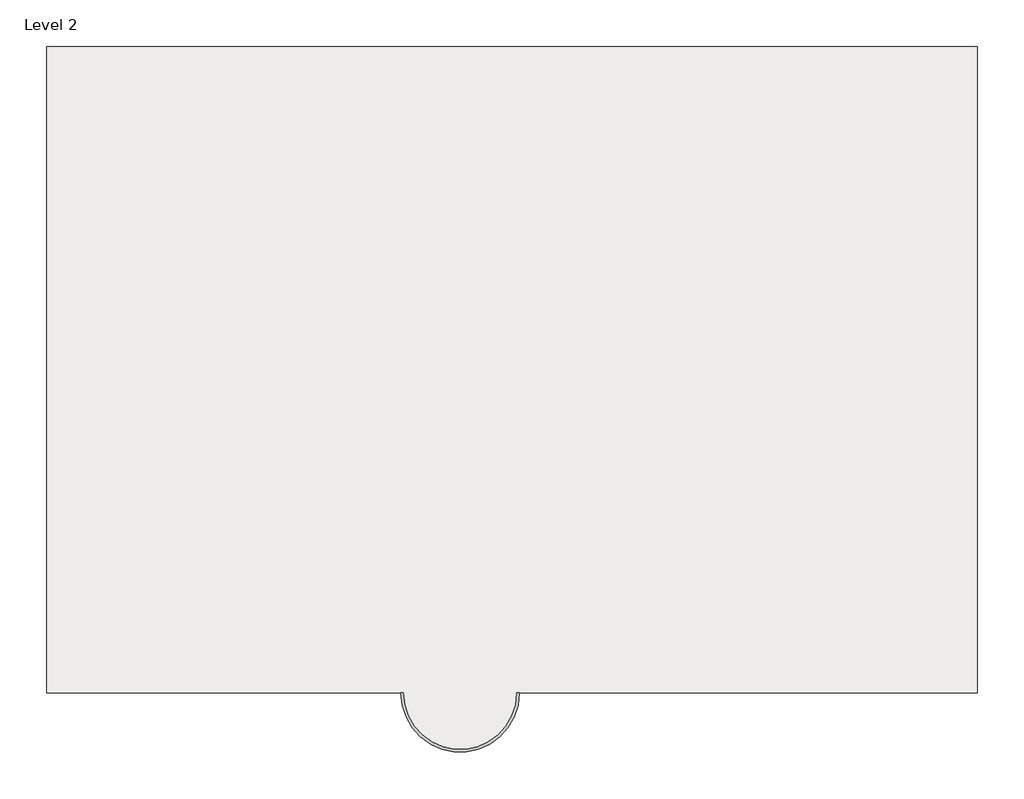
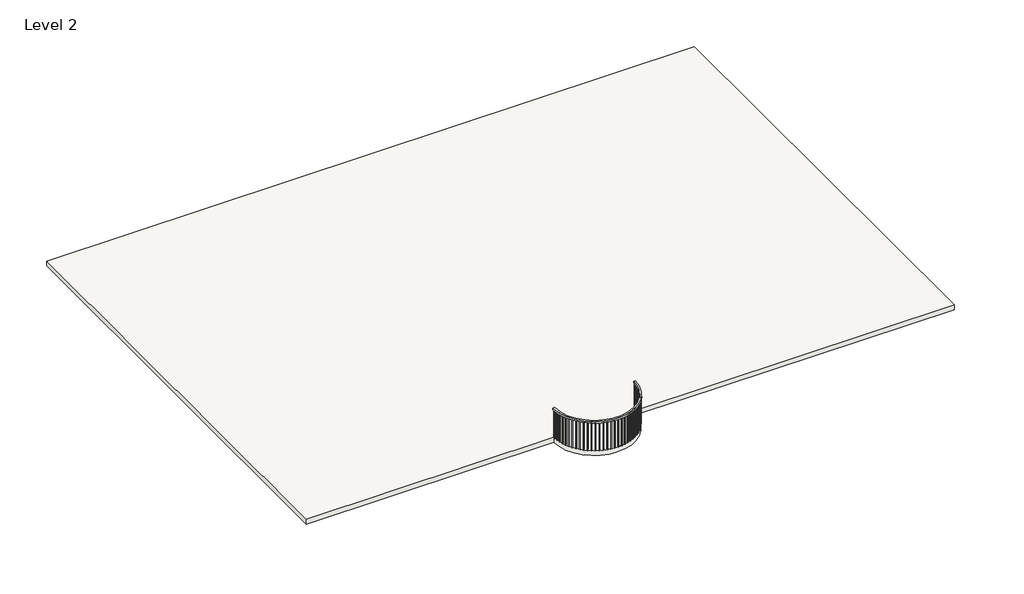
# One storey: 1 railing, 1 slab.
"""IFC4 building model written with IfcOpenShell, lengths in millimetres."""

from ifc_helpers import new_model, si_unit, point, frame, frame_2d, origin, place, context, project, spatial, polyline, circle_curve, trimmed, segment, composite_curve, outline, extrude, element, save

model = new_model("IFC4")

# Units and contexts
model_context = context("Model", 3, world=origin())
ifc_project = project(units=[si_unit("LENGTHUNIT", "METRE", prefix="MILLI")], contexts=[model_context])

# Site, building, storey
site = spatial("IfcSite", under=ifc_project)
building = spatial("IfcBuilding", under=site)
storey = spatial("IfcBuildingStorey", under=building, Name="Level 2", Elevation=3962.4)

# Railing
placement = place(None, origin())
element("IfcRailing", 1, ObjectType="Handrail - Rectangular", at=placement, inside=storey, context=model_context, shape_type="SweptSolid", body=[
    extrude(outline(composite_curve([segment(trimmed(circle_curve(frame_2d((-1741.9484006, -4605.2372669)), 1155.7), [point((-2897.6484006, -4605.2372669))], [point((-586.2484006, -4605.2372669))], True, "CARTESIAN"), True, "CONTINUOUS"), segment(polyline([(-586.2484006, -4605.2372669), (-535.4484006, -4605.2372669)]), True, "CONTINUOUS"), segment(trimmed(circle_curve(frame_2d((-1741.9484006, -4605.2372669)), 1206.5), [point((-535.4484006, -4605.2372669))], [point((-2948.4484006, -4605.2372669))], False, "CARTESIAN"), True, "CONTINUOUS"), segment(polyline([(-2948.4484006, -4605.2372669), (-2897.6484006, -4605.2372669)]), True, "CONTINUOUS")], self_intersect=False)), frame((0.0, 0.0, 4978.4), z_axis=(0.0, 0.0, 1.0), x_axis=(1.0, 0.0, 0.0)), (0.0, 0.0, 1.0), 50.8),
    extrude(outline(polyline([(-2911.9201765, -4667.2433123), (-2930.9510469, -4668.0968182), (-2931.8045528, -4649.0659478), (-2912.7736824, -4648.2124419), (-2911.9201765, -4667.2433123)])), frame((0.0, 0.0, 4114.8), z_axis=(0.0, 0.0, 1.0), x_axis=(1.0, 0.0, 0.0)), (0.0, 0.0, 1.0), 863.6),
    extrude(outline(polyline([(-2902.2668478, -4767.5326991), (-2921.1540209, -4770.0180949), (-2923.6394167, -4751.1309218), (-2904.7522436, -4748.645526), (-2902.2668478, -4767.5326991)])), frame((0.0, 0.0, 4114.8), z_axis=(0.0, 0.0, 1.0), x_axis=(1.0, 0.0, 0.0)), (0.0, 0.0, 1.0), 863.6),
    extrude(outline(polyline([(-2884.0328045, -4866.6218887), (-2902.636607, -4870.7207948), (-2906.7355131, -4852.1169922), (-2888.1317105, -4848.0180862), (-2884.0328045, -4866.6218887)])), frame((0.0, 0.0, 4114.8), z_axis=(0.0, 0.0, 1.0), x_axis=(1.0, 0.0, 0.0)), (0.0, 0.0, 1.0), 863.6),
    extrude(outline(polyline([(-2857.3528899, -4963.7781032), (-2875.5357443, -4969.4602074), (-2881.2178485, -4951.2773531), (-2863.0349942, -4945.5952488), (-2857.3528899, -4963.7781032)])), frame((0.0, 0.0, 4114.8), z_axis=(0.0, 0.0, 1.0), x_axis=(1.0, 0.0, 0.0)), (0.0, 0.0, 1.0), 863.6),
    extrude(outline(polyline([(-2822.4244058, -5058.2828588), (-2840.0518472, -5065.5061413), (-2847.2751296, -5047.8786999), (-2829.6476882, -5040.6554174), (-2822.4244058, -5058.2828588)])), frame((0.0, 0.0, 4114.8), z_axis=(0.0, 0.0, 1.0), x_axis=(1.0, 0.0, 0.0)), (0.0, 0.0, 1.0), 863.6),
    extrude(outline(polyline([(-2779.5056529, -5149.43728), (-2796.4473241, -5158.1483235), (-2805.1583676, -5141.2066524), (-2788.2166965, -5132.4956089), (-2779.5056529, -5149.43728)])), frame((0.0, 0.0, 4114.8), z_axis=(0.0, 0.0, 1.0), x_axis=(1.0, 0.0, 0.0)), (0.0, 0.0, 1.0), 863.6),
    extrude(outline(polyline([(-2728.9140215, -5236.5672672), (-2745.0446364, -5246.7016525), (-2755.1790216, -5230.5710376), (-2739.0484067, -5220.4366523), (-2728.9140215, -5236.5672672)])), frame((0.0, 0.0, 4114.8), z_axis=(0.0, 0.0, 1.0), x_axis=(1.0, 0.0, 0.0)), (0.0, 0.0, 1.0), 863.6),
    extrude(outline(polyline([(-2671.0236435, -5319.0284822), (-2686.223914, -5330.511264), (-2697.7066958, -5315.3109936), (-2682.5064253, -5303.8282118), (-2671.0236435, -5319.0284822)])), frame((0.0, 0.0, 4114.8), z_axis=(0.0, 0.0, 1.0), x_axis=(1.0, 0.0, 0.0)), (0.0, 0.0, 1.0), 863.6),
    extrude(outline(polyline([(-2606.2626264, -5396.211113), (-2620.4201443, -5408.9573746), (-2633.1664059, -5394.7998566), (-2619.0088879, -5382.053595), (-2606.2626264, -5396.211113)])), frame((0.0, 0.0, 4114.8), z_axis=(0.0, 0.0, 1.0), x_axis=(1.0, 0.0, 0.0)), (0.0, 0.0, 1.0), 863.6),
    extrude(outline(polyline([(-2535.1098866, -5467.5443835), (-2548.1199553, -5481.4598645), (-2562.0354363, -5468.4497957), (-2549.0253676, -5454.5343147), (-2535.1098866, -5467.5443835)])), frame((0.0, 0.0, 4114.8), z_axis=(0.0, 0.0, 1.0), x_axis=(1.0, 0.0, 0.0)), (0.0, 0.0, 1.0), 863.6),
    extrude(outline(polyline([(-2458.0916085, -5532.5007741), (-2469.8580167, -5547.4825677), (-2484.8398103, -5535.7161595), (-2473.0734021, -5520.7343659), (-2458.0916085, -5532.5007741)])), frame((0.0, 0.0, 4114.8), z_axis=(0.0, 0.0, 1.0), x_axis=(1.0, 0.0, 0.0)), (0.0, 0.0, 1.0), 863.6),
    extrude(outline(polyline([(-2375.777353, -5590.5999236), (-2386.2130864, -5606.5372373), (-2402.1504001, -5596.1015038), (-2391.7146666, -5580.1641902), (-2375.777353, -5590.5999236)])), frame((0.0, 0.0, 4114.8), z_axis=(0.0, 0.0, 1.0), x_axis=(1.0, 0.0, 0.0)), (0.0, 0.0, 1.0), 863.6),
    extrude(outline(polyline([(-2288.7758451, -5641.4121808), (-2297.8037302, -5658.1871559), (-2314.5787053, -5649.1592708), (-2305.5508202, -5632.3842957), (-2288.7758451, -5641.4121808)])), frame((0.0, 0.0, 4114.8), z_axis=(0.0, 0.0, 1.0), x_axis=(1.0, 0.0, 0.0)), (0.0, 0.0, 1.0), 863.6),
    extrude(outline(polyline([(-2197.730473, -5684.5617819), (-2205.2837473, -5702.0503652), (-2222.7723306, -5694.497091), (-2215.2190564, -5677.0085076), (-2197.730473, -5684.5617819)])), frame((0.0, 0.0, 4114.8), z_axis=(0.0, 0.0, 1.0), x_axis=(1.0, 0.0, 0.0)), (0.0, 0.0, 1.0), 863.6),
    extrude(outline(polyline([(-2103.3145299, -5719.7296297), (-2109.3373357, -5737.8024908), (-2127.4101969, -5731.779685), (-2121.387391, -5713.7068239), (-2103.3145299, -5719.7296297)])), frame((0.0, 0.0, 4114.8), z_axis=(0.0, 0.0, 1.0), x_axis=(1.0, 0.0, 0.0)), (0.0, 0.0, 1.0), 863.6),
    extrude(outline(polyline([(-2006.2262345, -5746.6556532), (-2010.6740325, -5765.1791408), (-2029.1975201, -5760.7313428), (-2024.7497221, -5742.2078552), (-2006.2262345, -5746.6556532)])), frame((0.0, 0.0, 4114.8), z_axis=(0.0, 0.0, 1.0), x_axis=(1.0, 0.0, 0.0)), (0.0, 0.0, 1.0), 863.6),
    extrude(outline(polyline([(-1907.1835682, -5765.1407308), (-1910.0234663, -5783.9778611), (-1928.8605966, -5781.137963), (-1926.0206985, -5762.3008327), (-1907.1835682, -5765.1407308)])), frame((0.0, 0.0, 4114.8), z_axis=(0.0, 0.0, 1.0), x_axis=(1.0, 0.0, 0.0)), (0.0, 0.0, 1.0), 863.6),
    extrude(outline(polyline([(-1806.9189651, -5775.0481627), (-1808.1299618, -5794.0596326), (-1827.1414317, -5792.8486358), (-1825.9304349, -5773.837166), (-1806.9189651, -5775.0481627)])), frame((0.0, 0.0, 4114.8), z_axis=(0.0, 0.0, 1.0), x_axis=(1.0, 0.0, 0.0)), (0.0, 0.0, 1.0), 863.6),
    extrude(outline(polyline([(-1706.1738957, -5776.3046821), (-1705.7470356, -5795.3498991), (-1724.7922526, -5795.7767592), (-1725.2191127, -5776.7315422), (-1706.1738957, -5776.3046821)])), frame((0.0, 0.0, 4114.8), z_axis=(0.0, 0.0, 1.0), x_axis=(1.0, 0.0, 0.0)), (0.0, 0.0, 1.0), 863.6),
    extrude(outline(polyline([(-1605.6933837, -5768.9009969), (-1603.6318234, -5787.839119), (-1622.5699456, -5789.9006793), (-1624.6315058, -5770.9625572), (-1605.6933837, -5768.9009969)])), frame((0.0, 0.0, 4114.8), z_axis=(0.0, 0.0, 1.0), x_axis=(1.0, 0.0, 0.0)), (0.0, 0.0, 1.0), 863.6),
    extrude(outline(polyline([(-1506.2204963, -5752.8918584), (-1502.5394814, -5771.5828356), (-1521.2304586, -5775.2638505), (-1524.9114735, -5756.5728733), (-1506.2204963, -5752.8918584)])), frame((0.0, 0.0, 4114.8), z_axis=(0.0, 0.0, 1.0), x_axis=(1.0, 0.0, 0.0)), (0.0, 0.0, 1.0), 863.6),
    extrude(outline(polyline([(-1408.4908492, -5728.3956563), (-1403.2176013, -5746.7012662), (-1421.5232112, -5751.9745142), (-1426.7964591, -5733.6689042), (-1408.4908492, -5728.3956563)])), frame((0.0, 0.0, 4114.8), z_axis=(0.0, 0.0, 1.0), x_axis=(1.0, 0.0, 0.0)), (0.0, 0.0, 1.0), 863.6),
    extrude(outline(polyline([(-1313.2271665, -5695.5935434), (-1306.400682, -5713.3784136), (-1324.1855522, -5720.2048981), (-1331.0120367, -5702.4200279), (-1313.2271665, -5695.5935434)])), frame((0.0, 0.0, 4114.8), z_axis=(0.0, 0.0, 1.0), x_axis=(1.0, 0.0, 0.0)), (0.0, 0.0, 1.0), 863.6),
    extrude(outline(polyline([(-1221.1339363, -5654.7280959), (-1212.804698, -5671.8607048), (-1229.9373069, -5680.1899431), (-1238.2665453, -5663.0573342), (-1221.1339363, -5654.7280959)])), frame((0.0, 0.0, 4114.8), z_axis=(0.0, 0.0, 1.0), x_axis=(1.0, 0.0, 0.0)), (0.0, 0.0, 1.0), 863.6),
    extrude(outline(polyline([(-1132.8922008, -5606.1015193), (-1123.1218044, -5622.4551689), (-1139.475454, -5632.2255652), (-1149.2458504, -5615.8719156), (-1132.8922008, -5606.1015193)])), frame((0.0, 0.0, 4114.8), z_axis=(0.0, 0.0, 1.0), x_axis=(1.0, 0.0, 0.0)), (0.0, 0.0, 1.0), 863.6),
    extrude(outline(polyline([(-1049.1545196, -5550.0734139), (-1038.0152187, -5565.5271667), (-1053.4689715, -5576.6664676), (-1064.6082724, -5561.2127148), (-1049.1545196, -5550.0734139)])), frame((0.0, 0.0, 4114.8), z_axis=(0.0, 0.0, 1.0), x_axis=(1.0, 0.0, 0.0)), (0.0, 0.0, 1.0), 863.6),
    extrude(outline(polyline([(-970.5401444, -5487.0581152), (-958.1143157, -5501.4976886), (-972.553889, -5513.9235174), (-984.9797178, -5499.483944), (-970.5401444, -5487.0581152)])), frame((0.0, 0.0, 4114.8), z_axis=(0.0, 0.0, 1.0), x_axis=(1.0, 0.0, 0.0)), (0.0, 0.0, 1.0), 863.6),
    extrude(outline(polyline([(-897.6304394, -5417.5216301), (-884.0099735, -5430.8402414), (-897.3285848, -5444.4607074), (-910.9490508, -5431.1420961), (-897.6304394, -5417.5216301)])), frame((0.0, 0.0, 4114.8), z_axis=(0.0, 0.0, 1.0), x_axis=(1.0, 0.0, 0.0)), (0.0, 0.0, 1.0), 863.6),
    extrude(outline(polyline([(-830.9645819, -5341.9781904), (-816.250204, -5354.0773467), (-828.3493603, -5368.7917246), (-843.0637382, -5356.6925683), (-830.9645819, -5341.9781904)])), frame((0.0, 0.0, 4114.8), z_axis=(0.0, 0.0, 1.0), x_axis=(1.0, 0.0, 0.0)), (0.0, 0.0, 1.0), 863.6),
    extrude(outline(polyline([(-771.035575, -5260.9864502), (-755.3361, -5271.7766766), (-766.1263264, -5287.4761516), (-781.8258014, -5276.6859252), (-771.035575, -5260.9864502)])), frame((0.0, 0.0, 4114.8), z_axis=(0.0, 0.0, 1.0), x_axis=(1.0, 0.0, 0.0)), (0.0, 0.0, 1.0), 863.6),
    extrude(outline(polyline([(-718.286602, -5175.1453546), (-701.7181297, -5184.5468558), (-711.1196309, -5201.1153282), (-727.6881032, -5191.713827), (-718.286602, -5175.1453546)])), frame((0.0, 0.0, 4114.8), z_axis=(0.0, 0.0, 1.0), x_axis=(1.0, 0.0, 0.0)), (0.0, 0.0, 1.0), 863.6),
    extrude(outline(polyline([(-673.1077488, -5085.0897103), (-655.7928053, -5093.032961), (-663.736056, -5110.3479045), (-681.0509995, -5102.4046539), (-673.1077488, -5085.0897103)])), frame((0.0, 0.0, 4114.8), z_axis=(0.0, 0.0, 1.0), x_axis=(1.0, 0.0, 0.0)), (0.0, 0.0, 1.0), 863.6),
    extrude(outline(polyline([(-635.8331193, -4991.4854912), (-617.899751, -4997.9117499), (-624.3260096, -5015.8451182), (-642.259378, -5009.4188595), (-635.8331193, -4991.4854912)])), frame((0.0, 0.0, 4114.8), z_axis=(0.0, 0.0, 1.0), x_axis=(1.0, 0.0, 0.0)), (0.0, 0.0, 1.0), 863.6),
    extrude(outline(polyline([(-606.7383644, -4895.0249134), (-588.319191, -4899.886657), (-593.1809346, -4918.3058304), (-611.600108, -4913.4440868), (-606.7383644, -4895.0249134)])), frame((0.0, 0.0, 4114.8), z_axis=(0.0, 0.0, 1.0), x_axis=(1.0, 0.0, 0.0)), (0.0, 0.0, 1.0), 863.6),
    extrude(outline(polyline([(-586.0386439, -4796.421316), (-567.2698777, -4799.6825913), (-570.531153, -4818.4513575), (-589.2999192, -4815.1900821), (-586.0386439, -4796.421316)])), frame((0.0, 0.0, 4114.8), z_axis=(0.0, 0.0, 1.0), x_axis=(1.0, 0.0, 0.0)), (0.0, 0.0, 1.0), 863.6),
    extrude(outline(polyline([(-573.887035, -4696.4038863), (-554.9074737, -4698.0405757), (-556.5441631, -4717.020137), (-575.5237244, -4715.3834476), (-573.887035, -4696.4038863)])), frame((0.0, 0.0, 4114.8), z_axis=(0.0, 0.0, 1.0), x_axis=(1.0, 0.0, 0.0)), (0.0, 0.0, 1.0), 863.6),
    extrude(outline(polyline([(-2913.4084896, -4624.2100402), (-2932.4578701, -4624.3636676), (-2932.6114975, -4605.314287), (-2913.5621169, -4605.1606597), (-2913.4084896, -4624.2100402)])), frame((0.0, 0.0, 4114.8), z_axis=(0.0, 0.0, 1.0), x_axis=(1.0, 0.0, 0.0)), (0.0, 0.0, 1.0), 863.6),
    extrude(outline(polyline([(-570.3346842, -4605.1606597), (-551.2853037, -4605.314287), (-551.438931, -4624.3636676), (-570.4883116, -4624.2100402), (-570.3346842, -4605.1606597)])), frame((0.0, 0.0, 4114.8), z_axis=(0.0, 0.0, 1.0), x_axis=(1.0, 0.0, 0.0)), (0.0, 0.0, 1.0), 863.6),
])

# Slab
element("IfcSlab", 2, ObjectType="6\" floor", at=placement, inside=storey, context=model_context, shape_type="SweptSolid", body=[
    extrude(outline(composite_curve([segment(polyline([(-10171.1852284, -4605.2372669), (-10171.1852284, 8577.3627331), (8802.6147716, 8577.3627331), (8802.6147716, -4605.2372669), (-560.8484006, -4605.2372669)]), True, "CONTINUOUS"), segment(trimmed(circle_curve(frame_2d((-1741.9484006, -4605.2372669)), 1181.1), [point((-560.8484006, -4605.2372669))], [point((-2923.0484006, -4605.2372669))], False, "CARTESIAN"), True, "CONTINUOUS"), segment(polyline([(-2923.0484006, -4605.2372669), (-10171.1852284, -4605.2372669)]), True, "CONTINUOUS")], self_intersect=False)), frame((0.0, 0.0, 3962.4), z_axis=(0.0, 0.0, 1.0), x_axis=(1.0, 0.0, 0.0)), (0.0, 0.0, 1.0), 152.4),
])

save(model, "model.ifc")

# Revit data of these elements
# Type "Handrail - Rectangular"
#   Assembly Code = "C2010400"
#   built-in parameter 1008612 = 0.0416667 (stored number, unit not read)
#   built-in parameter 1008611 = 0.0416667 (stored number, unit not read)
#   built-in parameter 1008609 = 0.333333 (stored number, unit not read)
#   built-in parameter 1008604 = 0.166667 (stored number, unit not read)
#   built-in parameter 1008603 = 0.166667 (stored number, unit not read)
#   Railing Height = 3' - 0"
#   built-in parameter 1008630 = 2
#   built-in parameter 1008610 = 2
#   built-in parameter 1008618 = Baluster - Square : 3/4"
# Type "6\" floor"
#   Assembly Code = "B1010"
#   Function = 0
#   Layers, outside or top first: 0' - 6" "Wall" (function 1)
# Element 1 (IfcRailing, "Handrail - Rectangular")
#   built-in parameter 1008621 = 0.5 (stored number, unit not read)
#   Phase Created = New Construction
#   Materials on its faces: "railing"
# Element 2 (IfcSlab, "6\" floor")
#   built-in parameter 1001955 = -1.5708 (stored number, unit not read)
#   Height Offset From Level = 0' - 6"
#   Phase Created = New Construction
#   Materials on its faces: "Wall"
# Materials
#   "Wall": class "Generic", colour RGB 120 120 120, transparency 0, Cost = 0
#   "railing": class "Generic", colour RGB 120 120 120, transparency 0, Cost = 0
